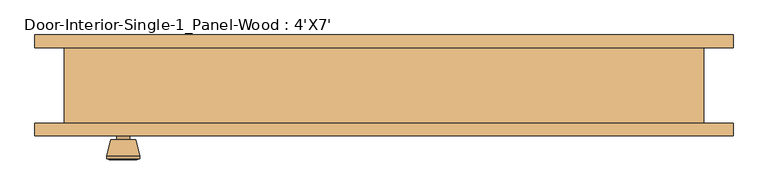
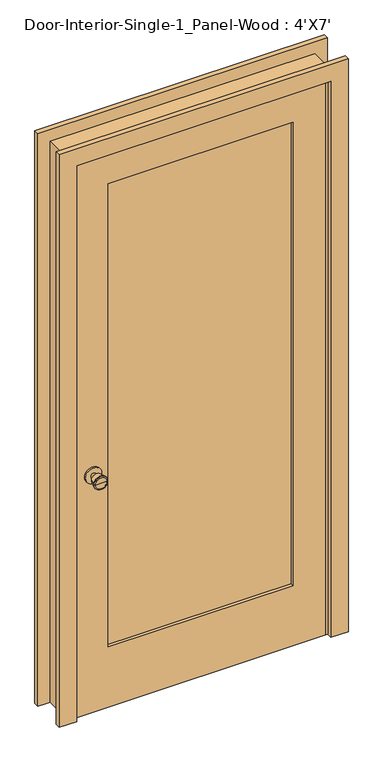
"""IFC4 building model written with IfcOpenShell, lengths in millimetres: door geometry, Door-Interior-Single-1_Panel-Wood : 4'X7'."""

from ifc_helpers import new_model, si_unit, point, frame, frame_2d, origin, place, context, project, spatial, polyline, circle_curve, trimmed, segment, composite_curve, outline, extrude, faceted_brep, source, transform, mapped, element, save
from ifc_brep_helpers import plane_surface, cylinder_surface, revolved_surface, advanced_brep


def door_interior_single_1_panel_wood_4_x7_a3feeac7(model_context):
    return source(origin(), model_context, "Body", "SolidModel", [
        advanced_brep(
        [(-393.7, -13.05, 914.4), (-403.7, -13.05, 914.4), (-383.7, -13.05, 914.4), (-373.2241324, 35.95, 914.4), (-414.1758676, 35.95, 914.4), (-393.7, 35.95, 914.4), (-368.7, 34.1221319, 914.4), (-418.7, 34.1221319, 914.4), (-368.7, 30.6584537, 914.4), (-418.7, 30.6584537, 914.4), (-375.063764, 5.95, 914.4), (-412.336236, 5.95, 914.4), (-383.7, 5.95, 914.4), (-403.7, 5.95, 914.4)],
        [
            (0, 1),
            (1, 2, circle_curve(frame((-393.7, -13.05, 914.4), z_axis=(0.0, -1.0, 0.0), x_axis=(-1.0, 0.0, 0.0)), 10.0)),
            (2, 0),
            (2, 1, circle_curve(frame((-393.7, -13.05, 914.4), z_axis=(0.0, -1.0, 0.0), x_axis=(-1.0, 0.0, 0.0)), 10.0)),
            (3, 4, circle_curve(frame((-393.7, 35.95, 914.4), z_axis=(0.0, 1.0, 0.0), x_axis=(-1.0, 0.0, 0.0)), 20.4758676)),
            (4, 5),
            (5, 3),
            (4, 3, circle_curve(frame((-393.7, 35.95, 914.4), z_axis=(0.0, 1.0, 0.0), x_axis=(-1.0, 0.0, 0.0)), 20.4758676)),
            (6, 7, circle_curve(frame((-393.7, 34.1221319, 914.4), z_axis=(0.0, 1.0, 0.0), x_axis=(-1.0, 0.0, 0.0)), 25.0)),
            (7, 4),
            (3, 6),
            (7, 6, circle_curve(frame((-393.7, 34.1221319, 914.4), z_axis=(0.0, 1.0, 0.0), x_axis=(-1.0, 0.0, 0.0)), 25.0)),
            (8, 9, circle_curve(frame((-393.7, 30.6584537, 914.4), z_axis=(0.0, 1.0, 0.0), x_axis=(-1.0, 0.0, 0.0)), 25.0)),
            (9, 7),
            (6, 8),
            (9, 8, circle_curve(frame((-393.7, 30.6584537, 914.4), z_axis=(0.0, 1.0, 0.0), x_axis=(-1.0, 0.0, 0.0)), 25.0)),
            (10, 11, circle_curve(frame((-393.7, 5.95, 914.4), z_axis=(0.0, 1.0, 0.0), x_axis=(-1.0, 0.0, 0.0)), 18.636236)),
            (11, 9),
            (8, 10),
            (11, 10, circle_curve(frame((-393.7, 5.95, 914.4), z_axis=(0.0, 1.0, 0.0), x_axis=(-1.0, 0.0, 0.0)), 18.636236)),
            (12, 13, circle_curve(frame((-393.7, 5.95, 914.4), z_axis=(0.0, 1.0, 0.0), x_axis=(-1.0, 0.0, 0.0)), 10.0)),
            (13, 11),
            (10, 12),
            (13, 12, circle_curve(frame((-393.7, 5.95, 914.4), z_axis=(0.0, 1.0, 0.0), x_axis=(-1.0, 0.0, 0.0)), 10.0)),
            (1, 13),
            (12, 2),
        ],
        [
            plane_surface(frame((-393.7, -13.05, 914.4), z_axis=(0.0, -1.0, 0.0), x_axis=(-1.0, 0.0, 0.0))),
            plane_surface(frame((-393.7, 35.95, 914.4), z_axis=(0.0, 1.0, 0.0), x_axis=(-1.0, 0.0, 0.0))),
            revolved_surface(polyline([(-414.1758676, 35.95, 914.4), (-418.7, 34.1221319, 914.4)]), (-393.7, -13.05, 914.4), (0.0, -1.0, 0.0)),
            cylinder_surface(frame((-393.7, -13.05, 914.4), z_axis=(0.0, -1.0, 0.0), x_axis=(-1.0, 0.0, 0.0)), 25.0),
            revolved_surface(polyline([(-418.7, 30.6584537, 914.4), (-412.336236, 5.95, 914.4)]), (-393.7, -13.05, 914.4), (0.0, -1.0, 0.0)),
            plane_surface(frame((-393.7, 5.95, 914.4), z_axis=(0.0, -1.0, 0.0), x_axis=(-1.0, 0.0, 0.0))),
            cylinder_surface(frame((-393.7, -13.05, 914.4), z_axis=(0.0, -1.0, 0.0), x_axis=(-1.0, 0.0, 0.0)), 10.0),
        ],
        [
            (0, [[1, 2, 3]]),
            (0, [[-3, 4, -1]]),
            (1, [[5, 6, 7]]),
            (1, [[8, -7, -6]]),
            (2, [[9, 10, -5, 11]]),
            (2, [[12, -11, -8, -10]]),
            (3, [[13, 14, -9, 15]]),
            (3, [[16, -15, -12, -14]]),
            (4, [[17, 18, -13, 19]]),
            (4, [[20, -19, -16, -18]]),
            (5, [[21, 22, -17, 23]]),
            (5, [[24, -23, -20, -22]]),
            (6, [[-2, 25, -21, 26]]),
            (6, [[-4, -26, -24, -25]]),
        ],
    ),
        extrude(outline(composite_curve([segment(trimmed(circle_curve(frame_2d((914.4, -393.7)), 30.0), [point((914.4, -423.7))], [point((914.4, -363.7))], False, "CARTESIAN"), True, "CONTINUOUS"), segment(trimmed(circle_curve(frame_2d((914.4, -393.7)), 30.0), [point((914.4, -363.7))], [point((914.4, -423.7))], False, "CARTESIAN"), True, "CONTINUOUS")], self_intersect=False)), frame((0.0, -19.05, 0.0), z_axis=(0.0, 1.0, 0.0), x_axis=(0.0, 0.0, 1.0)), (0.0, 0.0, 1.0), 6.0),
        advanced_brep(
        [(-393.7, -59.975, 914.4), (-383.7, -59.975, 914.4), (-403.7, -59.975, 914.4), (-373.2241324, -108.975, 914.4), (-393.7, -108.975, 914.4), (-414.1758676, -108.975, 914.4), (-368.7, -107.1471319, 914.4), (-418.7, -107.1471319, 914.4), (-368.7, -103.6834537, 914.4), (-418.7, -103.6834537, 914.4), (-375.063764, -78.975, 914.4), (-412.336236, -78.975, 914.4), (-383.7, -78.975, 914.4), (-403.7, -78.975, 914.4)],
        [
            (0, 1),
            (1, 2, circle_curve(frame((-393.7, -59.975, 914.4), z_axis=(0.0, 1.0, 0.0), x_axis=(-1.0, 0.0, 0.0)), 10.0)),
            (2, 0),
            (2, 1, circle_curve(frame((-393.7, -59.975, 914.4), z_axis=(0.0, 1.0, 0.0), x_axis=(-1.0, 0.0, 0.0)), 10.0)),
            (3, 4),
            (4, 5),
            (5, 3, circle_curve(frame((-393.7, -108.975, 914.4), z_axis=(0.0, -1.0, 0.0), x_axis=(-1.0, 0.0, 0.0)), 20.4758676)),
            (3, 5, circle_curve(frame((-393.7, -108.975, 914.4), z_axis=(0.0, -1.0, 0.0), x_axis=(-1.0, 0.0, 0.0)), 20.4758676)),
            (6, 3),
            (5, 7),
            (7, 6, circle_curve(frame((-393.7, -107.1471319, 914.4), z_axis=(0.0, -1.0, 0.0), x_axis=(-1.0, 0.0, 0.0)), 25.0)),
            (6, 7, circle_curve(frame((-393.7, -107.1471319, 914.4), z_axis=(0.0, -1.0, 0.0), x_axis=(-1.0, 0.0, 0.0)), 25.0)),
            (8, 6),
            (7, 9),
            (9, 8, circle_curve(frame((-393.7, -103.6834537, 914.4), z_axis=(0.0, -1.0, 0.0), x_axis=(-1.0, 0.0, 0.0)), 25.0)),
            (8, 9, circle_curve(frame((-393.7, -103.6834537, 914.4), z_axis=(0.0, -1.0, 0.0), x_axis=(-1.0, 0.0, 0.0)), 25.0)),
            (10, 8),
            (9, 11),
            (11, 10, circle_curve(frame((-393.7, -78.975, 914.4), z_axis=(0.0, -1.0, 0.0), x_axis=(-1.0, 0.0, 0.0)), 18.636236)),
            (10, 11, circle_curve(frame((-393.7, -78.975, 914.4), z_axis=(0.0, -1.0, 0.0), x_axis=(-1.0, 0.0, 0.0)), 18.636236)),
            (12, 10),
            (11, 13),
            (13, 12, circle_curve(frame((-393.7, -78.975, 914.4), z_axis=(0.0, -1.0, 0.0), x_axis=(-1.0, 0.0, 0.0)), 10.0)),
            (12, 13, circle_curve(frame((-393.7, -78.975, 914.4), z_axis=(0.0, -1.0, 0.0), x_axis=(-1.0, 0.0, 0.0)), 10.0)),
            (1, 12),
            (13, 2),
        ],
        [
            plane_surface(frame((-393.7, -59.975, 914.4), z_axis=(0.0, 1.0, 0.0), x_axis=(-1.0, 0.0, 0.0))),
            plane_surface(frame((-393.7, -108.975, 914.4), z_axis=(0.0, -1.0, 0.0), x_axis=(-1.0, 0.0, 0.0))),
            revolved_surface(polyline([(-414.1758676, -108.975, 914.4), (-418.7, -107.1471319, 914.4)]), (-393.7, -59.975, 914.4), (0.0, 1.0, 0.0)),
            cylinder_surface(frame((-393.7, -59.975, 914.4), z_axis=(0.0, 1.0, 0.0), x_axis=(-1.0, 0.0, 0.0)), 25.0),
            revolved_surface(polyline([(-418.7, -103.6834537, 914.4), (-412.336236, -78.975, 914.4)]), (-393.7, -59.975, 914.4), (0.0, 1.0, 0.0)),
            plane_surface(frame((-393.7, -78.975, 914.4), z_axis=(0.0, 1.0, 0.0), x_axis=(-1.0, 0.0, 0.0))),
            cylinder_surface(frame((-393.7, -59.975, 914.4), z_axis=(0.0, 1.0, 0.0), x_axis=(-1.0, 0.0, 0.0)), 10.0),
        ],
        [
            (0, [[1, 2, 3]]),
            (0, [[-3, 4, -1]]),
            (1, [[5, 6, 7]]),
            (1, [[-6, -5, 8]]),
            (2, [[9, -7, 10, 11]]),
            (2, [[-10, -8, -9, 12]]),
            (3, [[13, -11, 14, 15]]),
            (3, [[-14, -12, -13, 16]]),
            (4, [[17, -15, 18, 19]]),
            (4, [[-18, -16, -17, 20]]),
            (5, [[21, -19, 22, 23]]),
            (5, [[-22, -20, -21, 24]]),
            (6, [[25, -23, 26, -2]]),
            (6, [[-26, -24, -25, -4]]),
        ],
    ),
        extrude(outline(composite_curve([segment(trimmed(circle_curve(frame_2d((914.4, -393.7)), 30.0), [point((914.4, -423.7))], [point((914.4, -363.7))], False, "CARTESIAN"), True, "CONTINUOUS"), segment(trimmed(circle_curve(frame_2d((914.4, -393.7)), 30.0), [point((914.4, -363.7))], [point((914.4, -423.7))], False, "CARTESIAN"), True, "CONTINUOUS")], self_intersect=False)), frame((0.0, -59.975, 0.0), z_axis=(0.0, 1.0, 0.0), x_axis=(0.0, 0.0, 1.0)), (0.0, 0.0, 1.0), 6.0),
        faceted_brep([(482.6, -53.975, 0.0), (457.2, -53.975, 0.0), (457.2, -19.05, 0.0), (444.5, -19.05, 0.0), (444.5, 15.875, 0.0), (457.2, 15.875, 0.0), (457.2, 60.325, 0.0), (482.6, 60.325, 0.0), (482.6, 60.325, 2159.0), (482.6, -53.975, 2159.0), (457.2, 60.325, 2133.6), (-457.2, 60.325, 2133.6), (-457.2, 60.325, 0.0), (-482.6, 60.325, 0.0), (-482.6, 60.325, 2159.0), (457.2, 15.875, 2133.6), (444.5, 15.875, 2120.9), (-444.5, 15.875, 2120.9), (-444.5, 15.875, 0.0), (-457.2, 15.875, 0.0), (-457.2, 15.875, 2133.6), (444.5, -19.05, 2120.9), (457.2, -19.05, 2133.6), (-457.2, -19.05, 2133.6), (-457.2, -19.05, 0.0), (-444.5, -19.05, 0.0), (-444.5, -19.05, 2120.9), (457.2, -53.975, 2133.6), (-482.6, -53.975, 2159.0), (-482.6, -53.975, 0.0), (-457.2, -53.975, 0.0), (-457.2, -53.975, 2133.6)], [[[0, 1, 2, 3, 4, 5, 6, 7]], [[7, 8, 9, 0]], [[6, 10, 11, 12, 13, 14, 8, 7]], [[5, 15, 10, 6]], [[4, 16, 17, 18, 19, 20, 15, 5]], [[3, 21, 16, 4]], [[2, 22, 23, 24, 25, 26, 21, 3]], [[1, 27, 22, 2]], [[0, 9, 28, 29, 30, 31, 27, 1]], [[8, 14, 28, 9]], [[15, 20, 11, 10]], [[21, 26, 17, 16]], [[27, 31, 23, 22]], [[29, 13, 12, 19, 18, 25, 24, 30]], [[14, 13, 29, 28]], [[20, 19, 12, 11]], [[26, 25, 18, 17]], [[31, 30, 24, 23]]]),
        extrude(outline(polyline([(2133.6, -457.2), (0.0, -457.2), (0.0, 457.2), (2133.6, 457.2), (2133.6, -457.2)]), holes=[polyline([(2014.5375, -336.55), (2014.5375, 336.55), (231.775, 336.55), (231.775, -336.55), (2014.5375, -336.55)])]), frame((0.0, -53.975, 0.0), z_axis=(0.0, 1.0, 0.0), x_axis=(0.0, 0.0, 1.0)), (0.0, 0.0, 1.0), 34.925),
        extrude(outline(polyline([(336.55, -30.6916667), (336.55, -42.3333333), (-336.55, -42.3333333), (-336.55, -30.6916667), (336.55, -30.6916667)])), frame((0.0, 0.0, 231.775), z_axis=(0.0, 0.0, 1.0), x_axis=(1.0, 0.0, 0.0)), (0.0, 0.0, 1.0), 1782.7625),
        extrude(outline(polyline([(0.0, 527.05), (2203.45, 527.05), (2203.45, -527.05), (0.0, -527.05), (0.0, -463.55), (2139.95, -463.55), (2139.95, 463.55), (0.0, 463.55), (0.0, 527.05)])), frame((0.0, -73.025, 0.0), z_axis=(0.0, 1.0, 0.0), x_axis=(0.0, 0.0, 1.0)), (0.0, 0.0, 1.0), 19.05),
        extrude(outline(polyline([(0.0, 527.05), (2203.45, 527.05), (2203.45, -527.05), (0.0, -527.05), (0.0, -463.55), (2139.95, -463.55), (2139.95, 463.55), (0.0, 463.55), (0.0, 527.05)])), frame((0.0, 60.325, 0.0), z_axis=(0.0, 1.0, 0.0), x_axis=(0.0, 0.0, 1.0)), (0.0, 0.0, 1.0), 19.05),
    ])


if __name__ == "__main__":
    model = new_model("IFC4")
    model_context = context("Model", 3, world=origin())
    ifc_project = project(units=[si_unit("LENGTHUNIT", "METRE", prefix="MILLI")], contexts=[model_context])
    site = spatial("IfcSite", under=ifc_project)
    building = spatial("IfcBuilding", under=site)
    placement = place(None, origin())
    door_interior_single_1_panel_wood_4_x7_shape = door_interior_single_1_panel_wood_4_x7_a3feeac7(model_context)
    element("IfcDoor", 1, ObjectType="Door-Interior-Single-1_Panel-Wood : 4'X7'", at=placement, inside=building, context=model_context, shape_type="MappedRepresentation", body=[
        mapped(door_interior_single_1_panel_wood_4_x7_shape, transform((0.0, 0.0, 0.0), x_axis=(1.0, 0.0, 0.0), y_axis=(0.0, 1.0, 0.0), z_axis=(0.0, 0.0, 1.0))),
    ])
    save(model, "model.ifc")

# Revit data of these elements
# Type "Door-Interior-Single-1_Panel-Wood : 4'X7'"
#   Type Mark = "9"
#   Assembly Code = "C1020300"
#   Analytic Construction = "Wooden"
#   Top Rail = 0' - 4 11/16"
#   Thickness = 0' - 1 3/8"
#   Thermal Resistance (R) = 2.5876 (h·ft²·°F)/BTU
#   Swing Angle [instance default] = 90.00°
#   Stiles = 0' - 4 3/4"
#   Rough Width = 3' - 2"
#   Rough Height = 7' - 1"
#   Height = 7' - 0"
#   Width = 3' - 0"
#   Heat Transfer Coefficient (U) = 0.3865 BTU/(h·ft²·°F)
#   Bottom Rail = 0' - 9 1/8"
#   Trim Material = Cherry
#   Panel Material = Cherry
#   Frame Material = Cherry
#   Door Handle Material = Aluminum
#   Visual Light Transmittance = 0
#   Solar Heat Gain Coefficient = 0
#   Wall Closure = (empty or 0)
#   Function = (empty or 0)
# Element 1 (IfcDoor, "Door-Interior-Single-1_Panel-Wood : 4'X7'")
#   Materials on its faces: "Cherry", "Aluminum"
# Materials
#   "Cherry": class "Wood", colour RGB 226 177 128, transparency 0, Description = "Prunus Serotina", Cost = 0
#   "Aluminum": class "Metal", colour RGB 247 247 247, transparency 0, Description = "Aluminum 6061", Cost = 0
